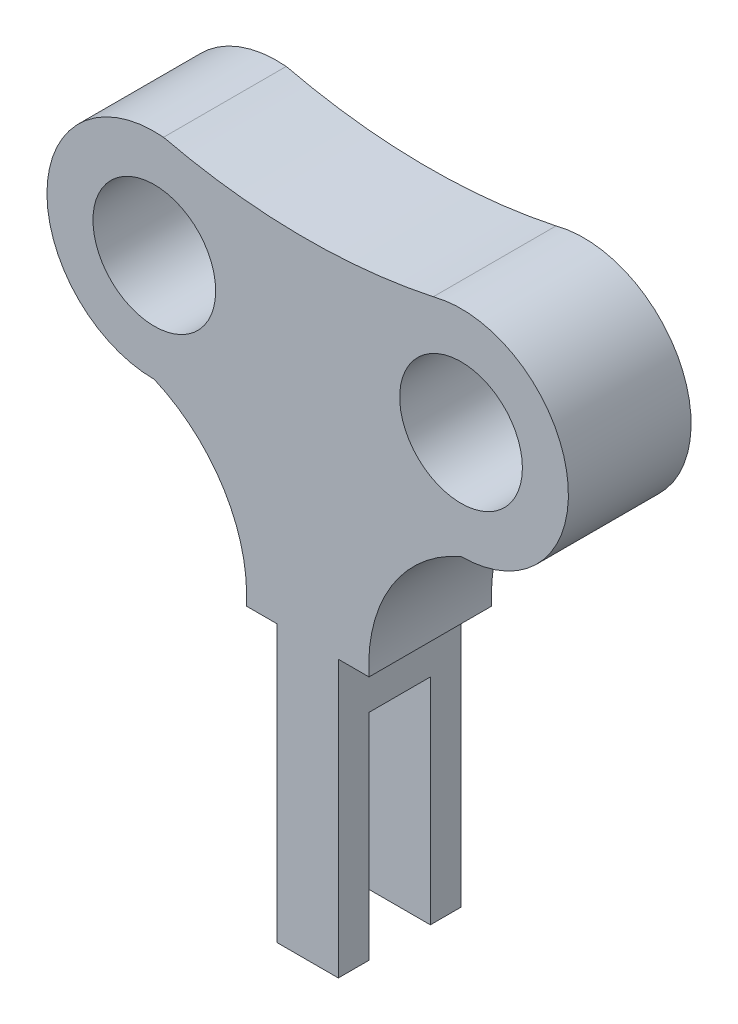
ISO-10303-21;
HEADER;
FILE_DESCRIPTION(('STEP AP214'),'2;1');
FILE_NAME('part.step','',(''),(''),'','','');
FILE_SCHEMA(('AUTOMOTIVE_DESIGN { 1 0 10303 214 1 1 1 1 }'));
ENDSEC;
DATA;
#1=APPLICATION_CONTEXT('core data for automotive mechanical design processes');
#2=APPLICATION_PROTOCOL_DEFINITION('international standard','automotive_design',2000,#1);
#3=PRODUCT_CONTEXT('',#1,'mechanical');
#4=PRODUCT('Part','Part','',(#3));
#5=PRODUCT_RELATED_PRODUCT_CATEGORY('part','',(#4));
#6=PRODUCT_DEFINITION_FORMATION('','',#4);
#7=PRODUCT_DEFINITION_CONTEXT('part definition',#1,'design');
#8=PRODUCT_DEFINITION('design','',#6,#7);
#9=PRODUCT_DEFINITION_SHAPE('','',#8);
#10=(LENGTH_UNIT() NAMED_UNIT(*) SI_UNIT(.MILLI.,.METRE.));
#11=(NAMED_UNIT(*) PLANE_ANGLE_UNIT() SI_UNIT($,.RADIAN.));
#12=(NAMED_UNIT(*) SI_UNIT($,.STERADIAN.) SOLID_ANGLE_UNIT());
#13=UNCERTAINTY_MEASURE_WITH_UNIT(LENGTH_MEASURE(1.E-05),#10,'distance_accuracy_value','');
#14=(GEOMETRIC_REPRESENTATION_CONTEXT(3) GLOBAL_UNCERTAINTY_ASSIGNED_CONTEXT((#13)) GLOBAL_UNIT_ASSIGNED_CONTEXT((#10,
#11,#12)) REPRESENTATION_CONTEXT('',''));
#15=CARTESIAN_POINT('',(0.,0.,0.));
#16=DIRECTION('',(0.,0.,1.));
#17=DIRECTION('',(1.,0.,0.));
#18=AXIS2_PLACEMENT_3D('',#15,#16,#17);
#19=CARTESIAN_POINT('',(20.,-87.,20.));
#20=DIRECTION('',(1.,0.,0.));
#21=DIRECTION('',(0.,0.,-1.));
#22=AXIS2_PLACEMENT_3D('',#19,#20,#21);
#23=PLANE('',#22);
#24=DIRECTION('',(0.,-1.,0.));
#25=VECTOR('',#24,1.);
#26=CARTESIAN_POINT('',(20.,-87.,5.));
#27=LINE('',#26,#25);
#28=CARTESIAN_POINT('',(20.,-52.,5.));
#29=VERTEX_POINT('',#28);
#30=CARTESIAN_POINT('',(20.,-87.,5.));
#31=VERTEX_POINT('',#30);
#32=EDGE_CURVE('E166',#29,#31,#27,.T.);
#33=ORIENTED_EDGE('',*,*,#32,.F.);
#34=DIRECTION('',(0.,0.,-1.));
#35=VECTOR('',#34,1.);
#36=CARTESIAN_POINT('',(20.,-52.,20.));
#37=LINE('',#36,#35);
#38=CARTESIAN_POINT('',(20.,-52.,15.));
#39=VERTEX_POINT('',#38);
#40=EDGE_CURVE('E242',#39,#29,#37,.T.);
#41=ORIENTED_EDGE('',*,*,#40,.F.);
#42=DIRECTION('',(0.,1.,0.));
#43=VECTOR('',#42,1.);
#44=CARTESIAN_POINT('',(20.,-87.,15.));
#45=LINE('',#44,#43);
#46=CARTESIAN_POINT('',(20.,-87.,15.));
#47=VERTEX_POINT('',#46);
#48=EDGE_CURVE('E238',#47,#39,#45,.T.);
#49=ORIENTED_EDGE('',*,*,#48,.F.);
#50=DIRECTION('',(0.,0.,-1.));
#51=VECTOR('',#50,1.);
#52=CARTESIAN_POINT('',(20.,-87.,20.));
#53=LINE('',#52,#51);
#54=CARTESIAN_POINT('',(20.,-87.,20.));
#55=VERTEX_POINT('',#54);
#56=EDGE_CURVE('E198',#55,#47,#53,.T.);
#57=ORIENTED_EDGE('',*,*,#56,.F.);
#58=DIRECTION('',(0.,-1.,0.));
#59=VECTOR('',#58,1.);
#60=CARTESIAN_POINT('',(20.,-87.,20.));
#61=LINE('',#60,#59);
#62=CARTESIAN_POINT('',(20.,-42.,20.));
#63=VERTEX_POINT('',#62);
#64=EDGE_CURVE('E226',#63,#55,#61,.T.);
#65=ORIENTED_EDGE('',*,*,#64,.F.);
#66=DIRECTION('',(0.,0.,-1.));
#67=VECTOR('',#66,1.);
#68=CARTESIAN_POINT('',(20.,-42.,20.));
#69=LINE('',#68,#67);
#70=CARTESIAN_POINT('',(20.,-42.,0.));
#71=VERTEX_POINT('',#70);
#72=EDGE_CURVE('E200',#63,#71,#69,.T.);
#73=ORIENTED_EDGE('',*,*,#72,.T.);
#74=DIRECTION('',(0.,-1.,0.));
#75=VECTOR('',#74,1.);
#76=CARTESIAN_POINT('',(20.,-87.,0.));
#77=LINE('',#76,#75);
#78=CARTESIAN_POINT('',(20.,-87.,0.));
#79=VERTEX_POINT('',#78);
#80=EDGE_CURVE('E174',#71,#79,#77,.T.);
#81=ORIENTED_EDGE('',*,*,#80,.T.);
#82=EDGE_CURVE('E193',#31,#79,#53,.T.);
#83=ORIENTED_EDGE('',*,*,#82,.F.);
#84=EDGE_LOOP('',(#33,#41,#49,#57,#65,#73,#81,#83));
#85=FACE_BOUND('',#84,.T.);
#86=ADVANCED_FACE('F44',(#85),#23,.F.);
#87=CARTESIAN_POINT('',(25.,-87.,20.));
#88=DIRECTION('',(0.,1.,0.));
#89=DIRECTION('',(0.,0.,1.));
#90=AXIS2_PLACEMENT_3D('',#87,#88,#89);
#91=PLANE('',#90);
#92=DIRECTION('',(1.,0.,0.));
#93=VECTOR('',#92,1.);
#94=CARTESIAN_POINT('',(10.,-87.,5.));
#95=LINE('',#94,#93);
#96=CARTESIAN_POINT('',(30.,-87.,5.));
#97=VERTEX_POINT('',#96);
#98=EDGE_CURVE('E247',#31,#97,#95,.T.);
#99=ORIENTED_EDGE('',*,*,#98,.F.);
#100=ORIENTED_EDGE('',*,*,#82,.T.);
#101=DIRECTION('',(1.,0.,0.));
#102=VECTOR('',#101,1.);
#103=CARTESIAN_POINT('',(25.,-87.,0.));
#104=LINE('',#103,#102);
#105=CARTESIAN_POINT('',(30.,-87.,0.));
#106=VERTEX_POINT('',#105);
#107=EDGE_CURVE('E180',#79,#106,#104,.T.);
#108=ORIENTED_EDGE('',*,*,#107,.T.);
#109=DIRECTION('',(0.,0.,-1.));
#110=VECTOR('',#109,1.);
#111=CARTESIAN_POINT('',(30.,-87.,20.));
#112=LINE('',#111,#110);
#113=EDGE_CURVE('E192',#97,#106,#112,.T.);
#114=ORIENTED_EDGE('',*,*,#113,.F.);
#115=EDGE_LOOP('',(#99,#100,#108,#114));
#116=FACE_BOUND('',#115,.T.);
#117=ADVANCED_FACE('F303',(#116),#91,.F.);
#118=DIRECTION('',(1.,0.,0.));
#119=VECTOR('',#118,1.);
#120=CARTESIAN_POINT('',(10.,-87.,15.));
#121=LINE('',#120,#119);
#122=CARTESIAN_POINT('',(30.,-87.,15.));
#123=VERTEX_POINT('',#122);
#124=EDGE_CURVE('E251',#47,#123,#121,.T.);
#125=ORIENTED_EDGE('',*,*,#124,.T.);
#126=CARTESIAN_POINT('',(30.,-87.,20.));
#127=VERTEX_POINT('',#126);
#128=EDGE_CURVE('E194',#127,#123,#112,.T.);
#129=ORIENTED_EDGE('',*,*,#128,.F.);
#130=DIRECTION('',(1.,0.,0.));
#131=VECTOR('',#130,1.);
#132=CARTESIAN_POINT('',(25.,-87.,20.));
#133=LINE('',#132,#131);
#134=EDGE_CURVE('E228',#55,#127,#133,.T.);
#135=ORIENTED_EDGE('',*,*,#134,.F.);
#136=ORIENTED_EDGE('',*,*,#56,.T.);
#137=EDGE_LOOP('',(#125,#129,#135,#136));
#138=FACE_BOUND('',#137,.T.);
#139=ADVANCED_FACE('F313',(#138),#91,.F.);
#140=CARTESIAN_POINT('',(30.,-87.,20.));
#141=DIRECTION('',(-1.,0.,0.));
#142=DIRECTION('',(0.,0.,1.));
#143=AXIS2_PLACEMENT_3D('',#140,#141,#142);
#144=PLANE('',#143);
#145=DIRECTION('',(0.,-1.,0.));
#146=VECTOR('',#145,1.);
#147=CARTESIAN_POINT('',(30.,0.,5.));
#148=LINE('',#147,#146);
#149=CARTESIAN_POINT('',(30.,-52.,5.));
#150=VERTEX_POINT('',#149);
#151=EDGE_CURVE('E58',#150,#97,#148,.T.);
#152=ORIENTED_EDGE('',*,*,#151,.T.);
#153=ORIENTED_EDGE('',*,*,#113,.T.);
#154=DIRECTION('',(0.,1.,0.));
#155=VECTOR('',#154,1.);
#156=CARTESIAN_POINT('',(30.,-87.,0.));
#157=LINE('',#156,#155);
#158=CARTESIAN_POINT('',(30.,-42.,0.));
#159=VERTEX_POINT('',#158);
#160=EDGE_CURVE('E182',#106,#159,#157,.T.);
#161=ORIENTED_EDGE('',*,*,#160,.T.);
#162=DIRECTION('',(0.,0.,-1.));
#163=VECTOR('',#162,1.);
#164=CARTESIAN_POINT('',(30.,-42.,20.));
#165=LINE('',#164,#163);
#166=CARTESIAN_POINT('',(30.,-42.,20.));
#167=VERTEX_POINT('',#166);
#168=EDGE_CURVE('E156',#167,#159,#165,.T.);
#169=ORIENTED_EDGE('',*,*,#168,.F.);
#170=DIRECTION('',(0.,1.,0.));
#171=VECTOR('',#170,1.);
#172=CARTESIAN_POINT('',(30.,-87.,20.));
#173=LINE('',#172,#171);
#174=EDGE_CURVE('E145',#127,#167,#173,.T.);
#175=ORIENTED_EDGE('',*,*,#174,.F.);
#176=ORIENTED_EDGE('',*,*,#128,.T.);
#177=DIRECTION('',(0.,1.,0.));
#178=VECTOR('',#177,1.);
#179=CARTESIAN_POINT('',(30.,0.,15.));
#180=LINE('',#179,#178);
#181=CARTESIAN_POINT('',(30.,-52.,15.));
#182=VERTEX_POINT('',#181);
#183=EDGE_CURVE('E248',#123,#182,#180,.T.);
#184=ORIENTED_EDGE('',*,*,#183,.T.);
#185=DIRECTION('',(0.,0.,-1.));
#186=VECTOR('',#185,1.);
#187=CARTESIAN_POINT('',(30.,-52.,0.));
#188=LINE('',#187,#186);
#189=EDGE_CURVE('E259',#182,#150,#188,.T.);
#190=ORIENTED_EDGE('',*,*,#189,.T.);
#191=EDGE_LOOP('',(#152,#153,#161,#169,#175,#176,#184,#190));
#192=FACE_BOUND('',#191,.T.);
#193=ADVANCED_FACE('F324',(#192),#144,.F.);
#194=CARTESIAN_POINT('',(24.6667458056474,114.716007843484,20.));
#195=DIRECTION('',(0.,0.,-1.));
#196=DIRECTION('',(-1.,0.,0.));
#197=AXIS2_PLACEMENT_3D('',#194,#195,#196);
#198=CYLINDRICAL_SURFACE('',#197,100.);
#199=CARTESIAN_POINT('',(24.6667458056474,114.716007843484,0.));
#200=DIRECTION('',(0.,0.,-1.));
#201=DIRECTION('',(1.,0.,0.));
#202=AXIS2_PLACEMENT_3D('',#199,#200,#201);
#203=CIRCLE('',#202,100.);
#204=CARTESIAN_POINT('',(45.4753353118932,16.9049522170339,0.));
#205=VERTEX_POINT('',#204);
#206=CARTESIAN_POINT('',(1.50597800256521,17.4350804487903,0.));
#207=VERTEX_POINT('',#206);
#208=EDGE_CURVE('E164',#205,#207,#203,.T.);
#209=ORIENTED_EDGE('',*,*,#208,.T.);
#210=DIRECTION('',(0.,0.,-1.));
#211=VECTOR('',#210,1.);
#212=CARTESIAN_POINT('',(1.50597800256521,17.4350804487903,20.));
#213=LINE('',#212,#211);
#214=CARTESIAN_POINT('',(1.50597800256521,17.4350804487903,20.));
#215=VERTEX_POINT('',#214);
#216=EDGE_CURVE('E11',#215,#207,#213,.T.);
#217=ORIENTED_EDGE('',*,*,#216,.F.);
#218=CARTESIAN_POINT('',(24.6667458056474,114.716007843484,20.));
#219=DIRECTION('',(0.,0.,-1.));
#220=DIRECTION('',(1.,0.,0.));
#221=AXIS2_PLACEMENT_3D('',#218,#219,#220);
#222=CIRCLE('',#221,100.);
#223=CARTESIAN_POINT('',(45.4753353118932,16.9049522170339,20.));
#224=VERTEX_POINT('',#223);
#225=EDGE_CURVE('E190',#224,#215,#222,.T.);
#226=ORIENTED_EDGE('',*,*,#225,.F.);
#227=DIRECTION('',(0.,0.,-1.));
#228=VECTOR('',#227,1.);
#229=CARTESIAN_POINT('',(45.4753353118932,16.9049522170339,20.));
#230=LINE('',#229,#228);
#231=EDGE_CURVE('E161',#224,#205,#230,.T.);
#232=ORIENTED_EDGE('',*,*,#231,.T.);
#233=EDGE_LOOP('',(#209,#217,#226,#232));
#234=FACE_BOUND('',#233,.T.);
#235=ADVANCED_FACE('F50',(#234),#198,.F.);
#236=CARTESIAN_POINT('',(0.,0.,20.));
#237=DIRECTION('',(0.,0.,-1.));
#238=DIRECTION('',(-1.,0.,0.));
#239=AXIS2_PLACEMENT_3D('',#236,#237,#238);
#240=CYLINDRICAL_SURFACE('',#239,17.5);
#241=CARTESIAN_POINT('',(0.,0.,0.));
#242=DIRECTION('',(0.,0.,1.));
#243=DIRECTION('',(1.,0.,0.));
#244=AXIS2_PLACEMENT_3D('',#241,#242,#243);
#245=CIRCLE('',#244,17.5);
#246=CARTESIAN_POINT('',(1.90819582357449E-13,-17.5,0.));
#247=VERTEX_POINT('',#246);
#248=EDGE_CURVE('E169',#207,#247,#245,.T.);
#249=ORIENTED_EDGE('',*,*,#248,.T.);
#250=DIRECTION('',(0.,0.,-1.));
#251=VECTOR('',#250,1.);
#252=CARTESIAN_POINT('',(1.90819582357449E-13,-17.5,20.));
#253=LINE('',#252,#251);
#254=CARTESIAN_POINT('',(1.90819582357449E-13,-17.5,20.));
#255=VERTEX_POINT('',#254);
#256=EDGE_CURVE('E52',#255,#247,#253,.T.);
#257=ORIENTED_EDGE('',*,*,#256,.F.);
#258=CARTESIAN_POINT('',(0.,0.,20.));
#259=DIRECTION('',(0.,0.,1.));
#260=DIRECTION('',(1.,0.,0.));
#261=AXIS2_PLACEMENT_3D('',#258,#259,#260);
#262=CIRCLE('',#261,17.5);
#263=EDGE_CURVE('E116',#215,#255,#262,.T.);
#264=ORIENTED_EDGE('',*,*,#263,.F.);
#265=ORIENTED_EDGE('',*,*,#216,.T.);
#266=EDGE_LOOP('',(#249,#257,#264,#265));
#267=FACE_BOUND('',#266,.T.);
#268=ADVANCED_FACE('F317',(#267),#240,.T.);
#269=CARTESIAN_POINT('',(-9.95091951131418,-40.4342364354984,20.));
#270=DIRECTION('',(0.,0.,-1.));
#271=DIRECTION('',(-1.,0.,0.));
#272=AXIS2_PLACEMENT_3D('',#269,#270,#271);
#273=CYLINDRICAL_SURFACE('',#272,25.);
#274=CARTESIAN_POINT('',(-9.95091951131418,-40.4342364354984,0.));
#275=DIRECTION('',(0.,0.,-1.));
#276=DIRECTION('',(1.,0.,0.));
#277=AXIS2_PLACEMENT_3D('',#274,#275,#276);
#278=CIRCLE('',#277,25.);
#279=CARTESIAN_POINT('',(15.,-42.,0.));
#280=VERTEX_POINT('',#279);
#281=EDGE_CURVE('E171',#247,#280,#278,.T.);
#282=ORIENTED_EDGE('',*,*,#281,.T.);
#283=DIRECTION('',(0.,0.,-1.));
#284=VECTOR('',#283,1.);
#285=CARTESIAN_POINT('',(15.,-42.,20.));
#286=LINE('',#285,#284);
#287=CARTESIAN_POINT('',(15.,-42.,20.));
#288=VERTEX_POINT('',#287);
#289=EDGE_CURVE('E205',#288,#280,#286,.T.);
#290=ORIENTED_EDGE('',*,*,#289,.F.);
#291=CARTESIAN_POINT('',(-9.95091951131418,-40.4342364354984,20.));
#292=DIRECTION('',(0.,0.,-1.));
#293=DIRECTION('',(1.,0.,0.));
#294=AXIS2_PLACEMENT_3D('',#291,#292,#293);
#295=CIRCLE('',#294,25.);
#296=EDGE_CURVE('E209',#255,#288,#295,.T.);
#297=ORIENTED_EDGE('',*,*,#296,.F.);
#298=ORIENTED_EDGE('',*,*,#256,.T.);
#299=EDGE_LOOP('',(#282,#290,#297,#298));
#300=FACE_BOUND('',#299,.T.);
#301=ADVANCED_FACE('F208',(#300),#273,.F.);
#302=CARTESIAN_POINT('',(20.,-42.,20.));
#303=DIRECTION('',(0.,1.,0.));
#304=DIRECTION('',(0.,0.,1.));
#305=AXIS2_PLACEMENT_3D('',#302,#303,#304);
#306=PLANE('',#305);
#307=DIRECTION('',(1.,0.,0.));
#308=VECTOR('',#307,1.);
#309=CARTESIAN_POINT('',(20.,-42.,0.));
#310=LINE('',#309,#308);
#311=EDGE_CURVE('E172',#280,#71,#310,.T.);
#312=ORIENTED_EDGE('',*,*,#311,.T.);
#313=ORIENTED_EDGE('',*,*,#72,.F.);
#314=DIRECTION('',(1.,0.,0.));
#315=VECTOR('',#314,1.);
#316=CARTESIAN_POINT('',(20.,-42.,20.));
#317=LINE('',#316,#315);
#318=EDGE_CURVE('E229',#288,#63,#317,.T.);
#319=ORIENTED_EDGE('',*,*,#318,.F.);
#320=ORIENTED_EDGE('',*,*,#289,.T.);
#321=EDGE_LOOP('',(#312,#313,#319,#320));
#322=FACE_BOUND('',#321,.T.);
#323=ADVANCED_FACE('F218',(#322),#306,.F.);
#324=CARTESIAN_POINT('',(30.,-42.,20.));
#325=DIRECTION('',(0.,1.,0.));
#326=DIRECTION('',(0.,0.,1.));
#327=AXIS2_PLACEMENT_3D('',#324,#325,#326);
#328=PLANE('',#327);
#329=DIRECTION('',(1.,0.,0.));
#330=VECTOR('',#329,1.);
#331=CARTESIAN_POINT('',(30.,-42.,0.));
#332=LINE('',#331,#330);
#333=CARTESIAN_POINT('',(35.,-42.,0.));
#334=VERTEX_POINT('',#333);
#335=EDGE_CURVE('E153',#159,#334,#332,.T.);
#336=ORIENTED_EDGE('',*,*,#335,.T.);
#337=DIRECTION('',(0.,0.,-1.));
#338=VECTOR('',#337,1.);
#339=CARTESIAN_POINT('',(35.,-42.,20.));
#340=LINE('',#339,#338);
#341=CARTESIAN_POINT('',(35.,-42.,20.));
#342=VERTEX_POINT('',#341);
#343=EDGE_CURVE('E147',#342,#334,#340,.T.);
#344=ORIENTED_EDGE('',*,*,#343,.F.);
#345=DIRECTION('',(1.,0.,0.));
#346=VECTOR('',#345,1.);
#347=CARTESIAN_POINT('',(30.,-42.,20.));
#348=LINE('',#347,#346);
#349=EDGE_CURVE('E139',#167,#342,#348,.T.);
#350=ORIENTED_EDGE('',*,*,#349,.F.);
#351=ORIENTED_EDGE('',*,*,#168,.T.);
#352=EDGE_LOOP('',(#336,#344,#350,#351));
#353=FACE_BOUND('',#352,.T.);
#354=ADVANCED_FACE('F151',(#353),#328,.F.);
#355=CARTESIAN_POINT('',(59.9509195113142,-40.4342364354986,20.));
#356=DIRECTION('',(0.,0.,-1.));
#357=DIRECTION('',(-1.,0.,0.));
#358=AXIS2_PLACEMENT_3D('',#355,#356,#357);
#359=CYLINDRICAL_SURFACE('',#358,25.);
#360=CARTESIAN_POINT('',(59.9509195113142,-40.4342364354986,0.));
#361=DIRECTION('',(0.,0.,-1.));
#362=DIRECTION('',(-1.,0.,0.));
#363=AXIS2_PLACEMENT_3D('',#360,#361,#362);
#364=CIRCLE('',#363,25.);
#365=CARTESIAN_POINT('',(50.0000000000002,-17.5,0.));
#366=VERTEX_POINT('',#365);
#367=EDGE_CURVE('E184',#334,#366,#364,.T.);
#368=ORIENTED_EDGE('',*,*,#367,.T.);
#369=DIRECTION('',(0.,0.,-1.));
#370=VECTOR('',#369,1.);
#371=CARTESIAN_POINT('',(50.0000000000002,-17.5,20.));
#372=LINE('',#371,#370);
#373=CARTESIAN_POINT('',(50.0000000000002,-17.5,20.));
#374=VERTEX_POINT('',#373);
#375=EDGE_CURVE('E160',#374,#366,#372,.T.);
#376=ORIENTED_EDGE('',*,*,#375,.F.);
#377=CARTESIAN_POINT('',(59.9509195113142,-40.4342364354986,20.));
#378=DIRECTION('',(0.,0.,-1.));
#379=DIRECTION('',(-1.,0.,0.));
#380=AXIS2_PLACEMENT_3D('',#377,#378,#379);
#381=CIRCLE('',#380,25.);
#382=EDGE_CURVE('E143',#342,#374,#381,.T.);
#383=ORIENTED_EDGE('',*,*,#382,.F.);
#384=ORIENTED_EDGE('',*,*,#343,.T.);
#385=EDGE_LOOP('',(#368,#376,#383,#384));
#386=FACE_BOUND('',#385,.T.);
#387=ADVANCED_FACE('F157',(#386),#359,.F.);
#388=CARTESIAN_POINT('',(50.,0.,20.));
#389=DIRECTION('',(0.,0.,-1.));
#390=DIRECTION('',(-1.,0.,0.));
#391=AXIS2_PLACEMENT_3D('',#388,#389,#390);
#392=CYLINDRICAL_SURFACE('',#391,17.5);
#393=CARTESIAN_POINT('',(50.,0.,0.));
#394=DIRECTION('',(0.,0.,1.));
#395=DIRECTION('',(1.,0.,0.));
#396=AXIS2_PLACEMENT_3D('',#393,#394,#395);
#397=CIRCLE('',#396,17.5);
#398=EDGE_CURVE('E107',#366,#205,#397,.T.);
#399=ORIENTED_EDGE('',*,*,#398,.T.);
#400=ORIENTED_EDGE('',*,*,#231,.F.);
#401=CARTESIAN_POINT('',(50.,0.,20.));
#402=DIRECTION('',(0.,0.,1.));
#403=DIRECTION('',(1.,0.,0.));
#404=AXIS2_PLACEMENT_3D('',#401,#402,#403);
#405=CIRCLE('',#404,17.5);
#406=EDGE_CURVE('E66',#374,#224,#405,.T.);
#407=ORIENTED_EDGE('',*,*,#406,.F.);
#408=ORIENTED_EDGE('',*,*,#375,.T.);
#409=EDGE_LOOP('',(#399,#400,#407,#408));
#410=FACE_BOUND('',#409,.T.);
#411=ADVANCED_FACE('F289',(#410),#392,.T.);
#412=CARTESIAN_POINT('',(24.6667458056474,114.716007843484,20.));
#413=DIRECTION('',(0.,0.,1.));
#414=DIRECTION('',(1.,0.,0.));
#415=AXIS2_PLACEMENT_3D('',#412,#413,#414);
#416=PLANE('',#415);
#417=CARTESIAN_POINT('',(0.,0.,20.));
#418=DIRECTION('',(0.,0.,1.));
#419=DIRECTION('',(1.,0.,0.));
#420=AXIS2_PLACEMENT_3D('',#417,#418,#419);
#421=CIRCLE('',#420,10.);
#422=CARTESIAN_POINT('',(10.,0.,20.));
#423=VERTEX_POINT('',#422);
#424=EDGE_CURVE('E269',#423,#423,#421,.T.);
#425=ORIENTED_EDGE('',*,*,#424,.F.);
#426=EDGE_LOOP('',(#425));
#427=FACE_BOUND('',#426,.T.);
#428=CARTESIAN_POINT('',(50.,0.,20.));
#429=DIRECTION('',(0.,0.,1.));
#430=DIRECTION('',(1.,0.,0.));
#431=AXIS2_PLACEMENT_3D('',#428,#429,#430);
#432=CIRCLE('',#431,10.);
#433=CARTESIAN_POINT('',(60.,0.,20.));
#434=VERTEX_POINT('',#433);
#435=EDGE_CURVE('E262',#434,#434,#432,.T.);
#436=ORIENTED_EDGE('',*,*,#435,.F.);
#437=EDGE_LOOP('',(#436));
#438=FACE_BOUND('',#437,.T.);
#439=ORIENTED_EDGE('',*,*,#225,.T.);
#440=ORIENTED_EDGE('',*,*,#263,.T.);
#441=ORIENTED_EDGE('',*,*,#296,.T.);
#442=ORIENTED_EDGE('',*,*,#318,.T.);
#443=ORIENTED_EDGE('',*,*,#64,.T.);
#444=ORIENTED_EDGE('',*,*,#134,.T.);
#445=ORIENTED_EDGE('',*,*,#174,.T.);
#446=ORIENTED_EDGE('',*,*,#349,.T.);
#447=ORIENTED_EDGE('',*,*,#382,.T.);
#448=ORIENTED_EDGE('',*,*,#406,.T.);
#449=EDGE_LOOP('',(#439,#440,#441,#442,#443,#444,#445,#446,#447,#448));
#450=FACE_BOUND('',#449,.T.);
#451=ADVANCED_FACE('F136',(#427,#438,#450),#416,.T.);
#452=CARTESIAN_POINT('',(24.6667458056474,114.716007843484,0.));
#453=DIRECTION('',(0.,0.,1.));
#454=DIRECTION('',(1.,0.,0.));
#455=AXIS2_PLACEMENT_3D('',#452,#453,#454);
#456=PLANE('',#455);
#457=CARTESIAN_POINT('',(0.,0.,0.));
#458=DIRECTION('',(0.,0.,1.));
#459=DIRECTION('',(1.,0.,0.));
#460=AXIS2_PLACEMENT_3D('',#457,#458,#459);
#461=CIRCLE('',#460,10.);
#462=CARTESIAN_POINT('',(10.,0.,0.));
#463=VERTEX_POINT('',#462);
#464=EDGE_CURVE('E263',#463,#463,#461,.T.);
#465=ORIENTED_EDGE('',*,*,#464,.T.);
#466=EDGE_LOOP('',(#465));
#467=FACE_BOUND('',#466,.T.);
#468=CARTESIAN_POINT('',(50.,0.,0.));
#469=DIRECTION('',(0.,0.,1.));
#470=DIRECTION('',(1.,0.,0.));
#471=AXIS2_PLACEMENT_3D('',#468,#469,#470);
#472=CIRCLE('',#471,10.);
#473=CARTESIAN_POINT('',(60.,0.,0.));
#474=VERTEX_POINT('',#473);
#475=EDGE_CURVE('E270',#474,#474,#472,.T.);
#476=ORIENTED_EDGE('',*,*,#475,.T.);
#477=EDGE_LOOP('',(#476));
#478=FACE_BOUND('',#477,.T.);
#479=ORIENTED_EDGE('',*,*,#208,.F.);
#480=ORIENTED_EDGE('',*,*,#398,.F.);
#481=ORIENTED_EDGE('',*,*,#367,.F.);
#482=ORIENTED_EDGE('',*,*,#335,.F.);
#483=ORIENTED_EDGE('',*,*,#160,.F.);
#484=ORIENTED_EDGE('',*,*,#107,.F.);
#485=ORIENTED_EDGE('',*,*,#80,.F.);
#486=ORIENTED_EDGE('',*,*,#311,.F.);
#487=ORIENTED_EDGE('',*,*,#281,.F.);
#488=ORIENTED_EDGE('',*,*,#248,.F.);
#489=EDGE_LOOP('',(#479,#480,#481,#482,#483,#484,#485,#486,#487,#488));
#490=FACE_BOUND('',#489,.T.);
#491=ADVANCED_FACE('F212',(#467,#478,#490),#456,.F.);
#492=CARTESIAN_POINT('',(10.,0.,5.));
#493=DIRECTION('',(0.,0.,1.));
#494=DIRECTION('',(1.,0.,0.));
#495=AXIS2_PLACEMENT_3D('',#492,#493,#494);
#496=PLANE('',#495);
#497=ORIENTED_EDGE('',*,*,#32,.T.);
#498=ORIENTED_EDGE('',*,*,#98,.T.);
#499=ORIENTED_EDGE('',*,*,#151,.F.);
#500=DIRECTION('',(1.,0.,0.));
#501=VECTOR('',#500,1.);
#502=CARTESIAN_POINT('',(10.,-52.,5.));
#503=LINE('',#502,#501);
#504=EDGE_CURVE('E249',#29,#150,#503,.T.);
#505=ORIENTED_EDGE('',*,*,#504,.F.);
#506=EDGE_LOOP('',(#497,#498,#499,#505));
#507=FACE_BOUND('',#506,.T.);
#508=ADVANCED_FACE('F362',(#507),#496,.T.);
#509=CARTESIAN_POINT('',(10.,0.,15.));
#510=DIRECTION('',(0.,0.,-1.));
#511=DIRECTION('',(-1.,0.,0.));
#512=AXIS2_PLACEMENT_3D('',#509,#510,#511);
#513=PLANE('',#512);
#514=ORIENTED_EDGE('',*,*,#48,.T.);
#515=DIRECTION('',(1.,0.,0.));
#516=VECTOR('',#515,1.);
#517=CARTESIAN_POINT('',(10.,-52.,15.));
#518=LINE('',#517,#516);
#519=EDGE_CURVE('E246',#39,#182,#518,.T.);
#520=ORIENTED_EDGE('',*,*,#519,.T.);
#521=ORIENTED_EDGE('',*,*,#183,.F.);
#522=ORIENTED_EDGE('',*,*,#124,.F.);
#523=EDGE_LOOP('',(#514,#520,#521,#522));
#524=FACE_BOUND('',#523,.T.);
#525=ADVANCED_FACE('F298',(#524),#513,.T.);
#526=CARTESIAN_POINT('',(10.,-52.,0.));
#527=DIRECTION('',(0.,-1.,0.));
#528=DIRECTION('',(0.,0.,-1.));
#529=AXIS2_PLACEMENT_3D('',#526,#527,#528);
#530=PLANE('',#529);
#531=ORIENTED_EDGE('',*,*,#40,.T.);
#532=ORIENTED_EDGE('',*,*,#504,.T.);
#533=ORIENTED_EDGE('',*,*,#189,.F.);
#534=ORIENTED_EDGE('',*,*,#519,.F.);
#535=EDGE_LOOP('',(#531,#532,#533,#534));
#536=FACE_BOUND('',#535,.T.);
#537=ADVANCED_FACE('F295',(#536),#530,.T.);
#538=CARTESIAN_POINT('',(50.,0.,0.));
#539=DIRECTION('',(0.,0.,1.));
#540=DIRECTION('',(1.,0.,0.));
#541=AXIS2_PLACEMENT_3D('',#538,#539,#540);
#542=CYLINDRICAL_SURFACE('',#541,10.);
#543=ORIENTED_EDGE('',*,*,#475,.F.);
#544=EDGE_LOOP('',(#543));
#545=FACE_BOUND('',#544,.T.);
#546=ORIENTED_EDGE('',*,*,#435,.T.);
#547=EDGE_LOOP('',(#546));
#548=FACE_BOUND('',#547,.T.);
#549=ADVANCED_FACE('F281',(#545,#548),#542,.F.);
#550=CARTESIAN_POINT('',(0.,0.,0.));
#551=DIRECTION('',(0.,0.,1.));
#552=DIRECTION('',(1.,0.,0.));
#553=AXIS2_PLACEMENT_3D('',#550,#551,#552);
#554=CYLINDRICAL_SURFACE('',#553,10.);
#555=ORIENTED_EDGE('',*,*,#464,.F.);
#556=EDGE_LOOP('',(#555));
#557=FACE_BOUND('',#556,.T.);
#558=ORIENTED_EDGE('',*,*,#424,.T.);
#559=EDGE_LOOP('',(#558));
#560=FACE_BOUND('',#559,.T.);
#561=ADVANCED_FACE('F279',(#557,#560),#554,.F.);
#562=CLOSED_SHELL('',(#86,#117,#139,#193,#235,#268,#301,#323,#354,#387,#411,#451,#491,#508,#525,
#537,#549,#561));
#563=MANIFOLD_SOLID_BREP('B2',#562);
#564=ADVANCED_BREP_SHAPE_REPRESENTATION('',(#18,#563),#14);
#565=SHAPE_DEFINITION_REPRESENTATION(#9,#564);
ENDSEC;
END-ISO-10303-21;
